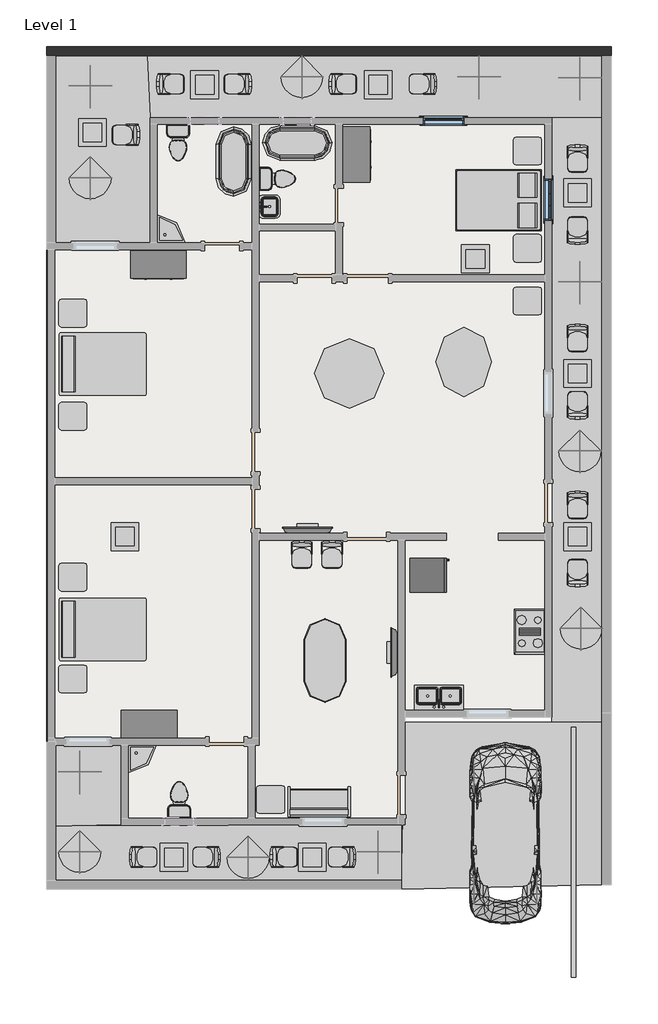
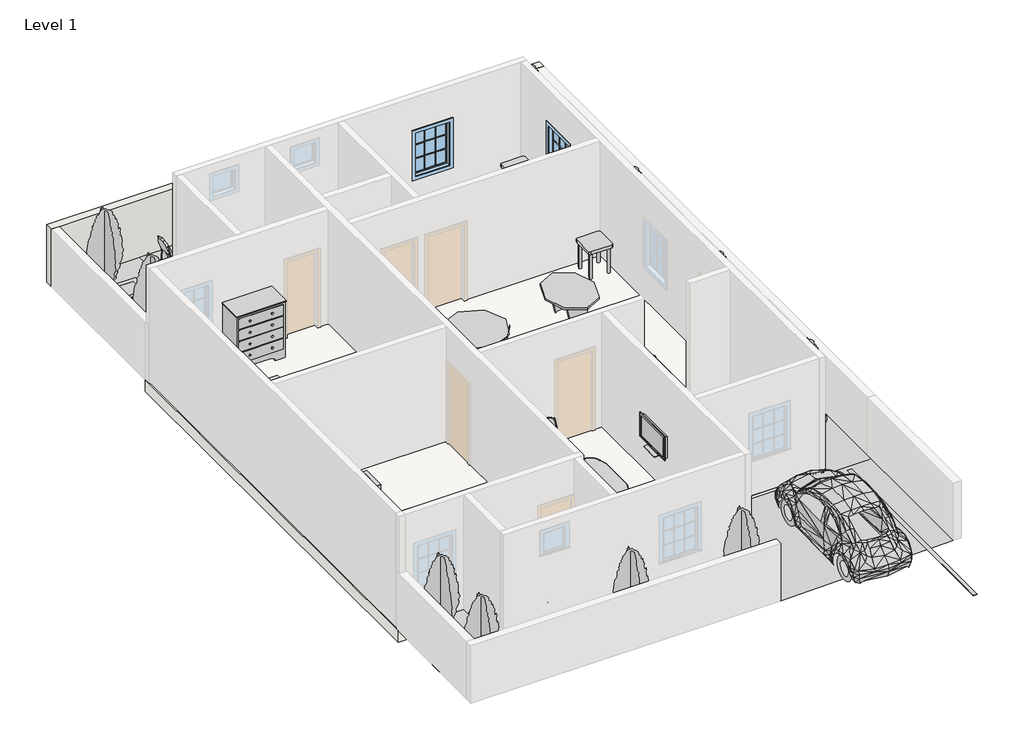
# One storey, part 2 of 2: 47 furniture elements, 12 geographic elements, 10 proxies, 9 flow terminals, 2 windows, 1 slab, 1 wall.
"""IFC4 building model written with IfcOpenShell, lengths in millimetres."""

from ifc_helpers import new_model, si_unit, frame, origin, place, context, project, spatial, polyline, outline, extrude, faceted_brep, triangles, transform, mapped, element, save
from components import proxy_bb1e6e30, parking_space_9_x_18_90_deg_b8b21359, rpc_beetle_rpc_beetle_3ce7ba48, proxy_a13a33b2, flow_terminal_bd5cdcf8, flow_terminal_a53be723, flow_terminal_62a433f7, toilet_domestic_3d_toilet_domestic_3d_f7549cf7, toilet_domestic_3d_toilet_domestic_3d_183bbd19, flow_terminal_b374fae2, furniture_c8abb964, furniture_0253826f, furniture_2babcf72, furniture_3d1d9cbc, furniture_22419f35, furniture_7a3aaa4f, furniture_b5c51a22, furniture_2c34a4f9, furniture_bbcc68ce, furniture_743965d2, furniture_bcf351fa, rpc_tree_conifer_chinese_juniper_7_1b9786cd, window_5c190c7e

model = new_model("IFC4")

# Units and contexts
model_context = context("Model", 3, world=origin())
ifc_project = project(units=[si_unit("LENGTHUNIT", "METRE", prefix="MILLI")], contexts=[model_context])

# Site, building, storey
site = spatial("IfcSite", under=ifc_project)
building = spatial("IfcBuilding", under=site)
storey = spatial("IfcBuildingStorey", under=building, Name="Level 1", Elevation=0.0)

# Proxies
placement = place(None, origin())
element("IfcBuildingElementProxy", 1, Name="Building Element Proxy", at=placement, inside=storey, context=model_context, shape_type="Tessellation", body=[
    triangles([(-15821.9726166, -3813.3326454, 0.0), (-14178.8159363, -3813.3326454, 0.0), (-14178.8159363, -5565.9329361, 0.0), (-15821.9726166, -5591.5796265, 0.0)], [[1, 4, 3], [3, 2, 1]], closed=False),
])
element("IfcBuildingElementProxy", 2, Name="Building Element Proxy", at=placement, inside=storey, context=model_context, shape_type="Tessellation", body=[
    triangles([(-13543.8163239, 7210.2674515, 0.0), (-15618.772229, 7210.2674515, 0.0), (-15618.772229, 11307.1063385, 0.0), (-13609.6855591, 11307.1063385, 0.0), (-13543.8163239, 9953.4668701, 0.0)], [[3, 2, 5], [3, 5, 4], [5, 2, 1]], closed=False),
])
element("IfcBuildingElementProxy", 3, Name="Building Element Proxy", at=placement, inside=storey, context=model_context, shape_type="Tessellation", body=[
    triangles([(-13528.6928284, 11219.4930817, 0.0), (-13558.0142944, 11217.5536652, 0.0), (-13543.8163239, 9953.4668701, 0.0), (-3629.9726166, 11225.4520203, 0.0), (-3629.9726166, 9951.5193146, 0.0), (-3629.9726166, 11307.1063385, 0.0), (-13621.8266785, 11226.9228607, 0.0), (-13607.6345215, 11233.7224457, 0.0), (-13588.6101013, 9952.7145905, 0.0), (-13611.7633392, 9956.2806519, 0.0), (-8604.8497696, 11307.1063385, 0.0), (-13593.9981445, 11307.1063385, 0.0)], [[2, 10, 3], [3, 10, 9], [10, 2, 7], [7, 8, 12], [8, 7, 2], [12, 8, 2], [2, 1, 12], [1, 3, 11], [5, 3, 9], [11, 3, 5], [3, 1, 2], [11, 4, 6], [4, 11, 5], [1, 11, 12]], closed=False),
])
element("IfcBuildingElementProxy", 4, Name="Building Element Proxy", at=placement, inside=storey, context=model_context, shape_type="Tessellation", body=[
    triangles([(-4730.0159363, 9953.4668701, 0.0), (-3629.9726166, 9959.906012, 0.0), (-4730.0159363, -3203.7326454, 0.0), (-3629.9726166, -3120.094146, 0.0), (-4724.8371826, -3329.7798935, 0.0), (-3629.9726166, -3346.9826225, 0.0)], [[4, 1, 3], [6, 3, 5], [4, 2, 1], [6, 4, 3]], closed=False),
])
element("IfcBuildingElementProxy", 5, Name="Building Element Proxy", at=placement, inside=storey, context=model_context, shape_type="Tessellation", body=[
    triangles([(-15618.772229, -5583.4679123, 0.0), (-14133.7047363, -5661.9735855, 0.0), (-15618.772229, -6777.6938553, 0.0), (-8032.0161301, -6777.6938553, 0.0), (-8032.0161301, -5565.9329361, 0.0)], [[1, 3, 2], [2, 4, 5], [4, 2, 3], [2, 5, 1]], closed=False),
])
element("IfcBuildingElementProxy", 6, Name="Building Element Proxy", at=placement, inside=storey, context=model_context, shape_type="Tessellation", body=[
    triangles([(-7762.1273712, -3550.9722061, 0.0), (-8032.0161301, -6980.8942429, 0.0), (-3629.9726166, -6879.2940491, 0.0), (-3629.9726166, -3374.0021942, 0.0), (-4730.0653519, -3327.8820442, 0.0), (-3629.9726166, -3308.4620087, 0.0), (-3629.9726166, -3320.1990829, 0.0), (-7860.2021988, -3759.4240173, 0.0), (-7955.8161301, -3309.578801, 0.0)], [[2, 8, 9], [1, 8, 5], [9, 1, 5], [1, 9, 8], [8, 2, 5], [3, 4, 5], [5, 6, 9], [5, 7, 6], [7, 5, 4], [3, 5, 2]], closed=False),
])
proxy_shape = proxy_bb1e6e30(model_context)
element("IfcBuildingElementProxy", 7, Name="Cook Top-4 Unit : 36\" x 20\"", ObjectType="Cook Top-4 Unit : 36\" x 20\"", at=placement, inside=storey, context=model_context, shape_type="MappedRepresentation", body=[
    mapped(proxy_shape, transform((-5212.6159934, -1324.1326671, 0.0), x_axis=(0.0, -1.0000000000000004, 0.0), y_axis=(1.0000000000000004, 0.0, 0.0), z_axis=(0.0, 0.0, 1.0))),
])
parking_space_9_x_18_90_deg_shape = parking_space_9_x_18_90_deg_b8b21359(model_context)
element("IfcBuildingElementProxy", 8, Name="Parking Space : 9' x 18' - 90 deg", ObjectType="Parking Space : 9' x 18' - 90 deg", at=placement, inside=storey, context=model_context, shape_type="MappedRepresentation", body=[
    mapped(parking_space_9_x_18_90_deg_shape, transform((-4247.4159934, -8911.2940071, 0.0), x_axis=(-1.0000000000000004, 0.0, 0.0), y_axis=(0.0, -1.0000000000000004, 0.0), z_axis=(0.0, 0.0, 1.0))),
])
rpc_beetle_rpc_beetle_shape = rpc_beetle_rpc_beetle_3ce7ba48(model_context)
element("IfcBuildingElementProxy", 9, Name="RPC Beetle : RPC Beetle", ObjectType="RPC Beetle : RPC Beetle", at=placement, inside=storey, context=model_context, shape_type="MappedRepresentation", body=[
    mapped(rpc_beetle_rpc_beetle_shape, transform((-5746.0159934, -6980.8940071, 0.0), x_axis=(1.0, 0.0, 0.0), y_axis=(0.0, 1.0, 0.0), z_axis=(0.0, 0.0, 1.0))),
])
proxy_2_shape = proxy_a13a33b2(model_context)
element("IfcBuildingElementProxy", 10, Name="Refrigerator : 30\" x 32\" RH", ObjectType="Refrigerator : 30\" x 32\" RH", at=placement, inside=storey, context=model_context, shape_type="MappedRepresentation", body=[
    mapped(proxy_2_shape, transform((-7455.7534934, -87.0816386, 0.0), x_axis=(0.0, 1.0000000000000002, 0.0), y_axis=(-1.0000000000000002, 0.0, 0.0), z_axis=(0.0, 0.0, 1.0))),
])

# Flow terminals
flow_terminal_shape = flow_terminal_bd5cdcf8(model_context)
element("IfcFlowTerminal", 11, ObjectType="Sink - Corner Floor : 24\"", at=placement, inside=storey, context=model_context, shape_type="MappedRepresentation", body=[
    mapped(flow_terminal_shape, transform((-13391.4159934, 7210.2673329, 609.6), x_axis=(1.0, 0.0, 0.0), y_axis=(0.0, 1.0, 0.0), z_axis=(0.0, 0.0, 1.0))),
])
element("IfcFlowTerminal", 12, ObjectType="Sink - Corner Floor : 24\"", at=placement, inside=storey, context=model_context, shape_type="MappedRepresentation", body=[
    mapped(flow_terminal_shape, transform((-14026.4159934, -3813.3326671, 609.6), x_axis=(0.0, -1.0000000000000009, 0.0), y_axis=(1.0000000000000009, 0.0, 0.0), z_axis=(0.0, 0.0, 1.0))),
])
flow_terminal_2_shape = flow_terminal_a53be723(model_context)
element("IfcFlowTerminal", 13, ObjectType="Sink Kitchen-Double : 42\" x 21\"", at=placement, inside=storey, context=model_context, shape_type="MappedRepresentation", body=[
    mapped(flow_terminal_2_shape, transform((-7190.8267528, -2769.587266, 0.0), x_axis=(-1.0000000000000004, 0.0, 0.0), y_axis=(0.0, -1.0000000000000004, 0.0), z_axis=(0.0, 0.0, 1.0))),
])
flow_terminal_3_shape = flow_terminal_62a433f7(model_context)
element("IfcFlowTerminal", 14, ObjectType="Sink Vanity-Square : 20\" x 18\"", at=placement, inside=storey, context=model_context, shape_type="MappedRepresentation", body=[
    mapped(flow_terminal_3_shape, transform((-10976.0705923, 7981.9780923, 0.0), x_axis=(0.0, 1.0, 0.0), y_axis=(-1.0, 0.0, 0.0), z_axis=(0.0, 0.0, 1.0))),
])
toilet_domestic_3d_toilet_domestic_3d_shape = toilet_domestic_3d_toilet_domestic_3d_f7549cf7(model_context)
toilet_domestic_3d_toilet_domestic_3d_2_shape = toilet_domestic_3d_toilet_domestic_3d_183bbd19(model_context)
element("IfcFlowTerminal", 15, ObjectType="Toilet-Domestic-3D : Toilet-Domestic-3D", at=placement, inside=storey, context=model_context, shape_type="MappedRepresentation", body=[
    mapped(toilet_domestic_3d_toilet_domestic_3d_shape, transform((-12934.2159934, 9306.3713055, 0.0), x_axis=(1.0, 0.0, 0.0), y_axis=(0.0, 1.0, 0.0), z_axis=(0.0, 0.0, 1.0))),
    mapped(toilet_domestic_3d_toilet_domestic_3d_2_shape, transform((-12934.2159934, 9306.3713055, 0.0), x_axis=(1.0, 0.0, 0.0), y_axis=(0.0, 1.0, 0.0), z_axis=(0.0, 0.0, 1.0))),
])
element("IfcFlowTerminal", 16, ObjectType="Toilet-Domestic-3D : Toilet-Domestic-3D", at=placement, inside=storey, context=model_context, shape_type="MappedRepresentation", body=[
    mapped(toilet_domestic_3d_toilet_domestic_3d_shape, transform((-10661.519966, 8607.2673329, 0.0), x_axis=(0.0, 1.0000000000000002, 0.0), y_axis=(-1.0000000000000002, 0.0, 0.0), z_axis=(0.0, 0.0, 1.0))),
    mapped(toilet_domestic_3d_toilet_domestic_3d_2_shape, transform((-10661.519966, 8607.2673329, 0.0), x_axis=(0.0, 1.0000000000000002, 0.0), y_axis=(-1.0000000000000002, 0.0, 0.0), z_axis=(0.0, 0.0, 1.0))),
])
element("IfcFlowTerminal", 17, ObjectType="Toilet-Domestic-3D : Toilet-Domestic-3D", at=placement, inside=storey, context=model_context, shape_type="MappedRepresentation", body=[
    mapped(toilet_domestic_3d_toilet_domestic_3d_shape, transform((-12908.8159934, -4918.8366398, 0.0), x_axis=(-0.9999999999999998, 0.0, 0.0), y_axis=(0.0, -0.9999999999999998, 0.0), z_axis=(0.0, 0.0, 1.0))),
    mapped(toilet_domestic_3d_toilet_domestic_3d_2_shape, transform((-12908.8159934, -4918.8366398, 0.0), x_axis=(-0.9999999999999998, 0.0, 0.0), y_axis=(0.0, -0.9999999999999998, 0.0), z_axis=(0.0, 0.0, 1.0))),
])
flow_terminal_4_shape = flow_terminal_b374fae2(model_context)
element("IfcFlowTerminal", 18, ObjectType="Tub-Free Standing-3D : 30\" x 60\"", at=placement, inside=storey, context=model_context, shape_type="MappedRepresentation", body=[
    mapped(flow_terminal_4_shape, transform((-11715.0159934, 8988.2673329, 0.0), x_axis=(1.0, 0.0, 0.0), y_axis=(0.0, 1.0, 0.0), z_axis=(0.0, 0.0, 1.0))),
])
element("IfcFlowTerminal", 19, ObjectType="Tub-Free Standing-3D : 30\" x 60\"", at=placement, inside=storey, context=model_context, shape_type="MappedRepresentation", body=[
    mapped(flow_terminal_4_shape, transform((-10318.0159934, 9394.6673329, 0.0), x_axis=(0.0, 1.0, 0.0), y_axis=(-1.0, 0.0, 0.0), z_axis=(0.0, 0.0, 1.0))),
])

# Furniture
furniture_shape = furniture_c8abb964(model_context)
element("IfcFurniture", 20, ObjectType="Bed-Box : Double 53\" x 74\"", at=placement, inside=storey, context=model_context, shape_type="MappedRepresentation", body=[
    mapped(furniture_shape, transform((-5663.9864852, 8476.5197919, 0.0), x_axis=(0.0, -1.0000000000000004, 0.0), y_axis=(1.0000000000000004, 0.0, 0.0), z_axis=(0.0, 0.0, 1.0))),
])
furniture_2_shape = furniture_0253826f(model_context)
element("IfcFurniture", 21, ObjectType="Bed-Standard : Double 54\" x 75\"", at=placement, inside=storey, context=model_context, shape_type="MappedRepresentation", body=[
    mapped(furniture_2_shape, transform((-14635.6677866, -1544.8211917, 0.0), x_axis=(0.0, 1.0000000000000002, 0.0), y_axis=(-1.0000000000000002, 0.0, 0.0), z_axis=(0.0, 0.0, 1.0))),
])
element("IfcFurniture", 22, ObjectType="Bed-Standard.0001 : Double 54\" x 75\"", at=placement, inside=storey, context=model_context, shape_type="MappedRepresentation", body=[
    mapped(furniture_2_shape, transform((-14635.6677866, 4271.7788083, 0.0), x_axis=(0.0, 1.0, 0.0), y_axis=(-1.0, 0.0, 0.0), z_axis=(0.0, 0.0, 1.0))),
])
furniture_3_shape = furniture_2babcf72(model_context)
element("IfcFurniture", 23, ObjectType="Dresser : 48\" x 60\" x 24\"", at=placement, inside=storey, context=model_context, shape_type="MappedRepresentation", body=[
    mapped(furniture_3_shape, transform((-9385.7789475, 9409.8605927, 0.0), x_axis=(0.0, 1.0, 0.0), y_axis=(-1.0, 0.0, 0.0), z_axis=(0.0, 0.0, 1.0))),
])
element("IfcFurniture", 24, ObjectType="Dresser : 48\" x 60\" x 24\"", at=placement, inside=storey, context=model_context, shape_type="MappedRepresentation", body=[
    mapped(furniture_3_shape, transform((-13096.8227336, 7090.830287, 0.0), x_axis=(1.0, 0.0, 0.0), y_axis=(0.0, 1.0, 0.0), z_axis=(0.0, 0.0, 1.0))),
])
element("IfcFurniture", 25, ObjectType="Dresser : 48\" x 60\" x 24\"", at=placement, inside=storey, context=model_context, shape_type="MappedRepresentation", body=[
    mapped(furniture_3_shape, transform((-13300.0227336, -2992.969713, 0.0), x_axis=(1.0, 0.0, 0.0), y_axis=(0.0, 1.0, 0.0), z_axis=(0.0, 0.0, 1.0))),
])
furniture_4_shape = furniture_3d1d9cbc(model_context)
element("IfcFurniture", 26, ObjectType="Seating-Auditorium : 18\" x 24\" x 30\"", at=placement, inside=storey, context=model_context, shape_type="MappedRepresentation", body=[
    mapped(furniture_4_shape, transform((-9395.2881245, 567.5427427, 0.0), x_axis=(-1.0000000000000002, 0.0, 0.0), y_axis=(0.0, -1.0000000000000002, 0.0), z_axis=(0.0, 0.0, 1.0))),
])
element("IfcFurniture", 27, ObjectType="Seating-Auditorium : 18\" x 24\" x 30\"", at=placement, inside=storey, context=model_context, shape_type="MappedRepresentation", body=[
    mapped(furniture_4_shape, transform((-10055.6881245, 567.5427427, 0.0), x_axis=(-1.0, 0.0, 0.0), y_axis=(0.0, -1.0, 0.0), z_axis=(0.0, 0.0, 1.0))),
])
element("IfcFurniture", 28, ObjectType="Seating-Auditorium : 18\" x 24\" x 30\"", at=placement, inside=storey, context=model_context, shape_type="MappedRepresentation", body=[
    mapped(furniture_4_shape, transform((-13899.6939644, -6108.9661382, 0.0), x_axis=(0.0, -1.0, 0.0), y_axis=(1.0, 0.0, 0.0), z_axis=(0.0, 0.0, 1.0))),
])
element("IfcFurniture", 29, ObjectType="Seating-Auditorium : 18\" x 24\" x 30\"", at=placement, inside=storey, context=model_context, shape_type="MappedRepresentation", body=[
    mapped(furniture_4_shape, transform((-12109.3405836, -6430.4218759, 0.0), x_axis=(0.0, 1.0, 0.0), y_axis=(-1.0, 0.0, 0.0), z_axis=(0.0, 0.0, 1.0))),
])
element("IfcFurniture", 30, ObjectType="Seating-Auditorium : 18\" x 24\" x 30\"", at=placement, inside=storey, context=model_context, shape_type="MappedRepresentation", body=[
    mapped(furniture_4_shape, transform((-10812.6914032, -6108.9661382, 0.0), x_axis=(0.0, -1.0000000000000004, 0.0), y_axis=(1.0000000000000004, 0.0, 0.0), z_axis=(0.0, 0.0, 1.0))),
])
element("IfcFurniture", 31, ObjectType="Seating-Auditorium : 18\" x 24\" x 30\"", at=placement, inside=storey, context=model_context, shape_type="MappedRepresentation", body=[
    mapped(furniture_4_shape, transform((-9137.5405836, -6430.4218759, 0.0), x_axis=(0.0, 1.0, 0.0), y_axis=(-1.0, 0.0, 0.0), z_axis=(0.0, 0.0, 1.0))),
])
element("IfcFurniture", 32, ObjectType="Seating-Auditorium : 18\" x 24\" x 30\"", at=placement, inside=storey, context=model_context, shape_type="MappedRepresentation", body=[
    mapped(furniture_4_shape, transform((-13879.4972948, 9411.739464, 0.0), x_axis=(0.0, 1.0000000000000002, 0.0), y_axis=(-1.0000000000000002, 0.0, 0.0), z_axis=(0.0, 0.0, 1.0))),
])
element("IfcFurniture", 33, ObjectType="Seating-Auditorium : 18\" x 24\" x 30\"", at=placement, inside=storey, context=model_context, shape_type="MappedRepresentation", body=[
    mapped(furniture_4_shape, transform((-13301.8914032, 10850.7952017, 0.0), x_axis=(0.0, -1.0000000000000004, 0.0), y_axis=(1.0000000000000004, 0.0, 0.0), z_axis=(0.0, 0.0, 1.0))),
])
element("IfcFurniture", 34, ObjectType="Seating-Auditorium : 18\" x 24\" x 30\"", at=placement, inside=storey, context=model_context, shape_type="MappedRepresentation", body=[
    mapped(furniture_4_shape, transform((-11423.5405836, 10529.339464, 0.0), x_axis=(0.0, 1.0, 0.0), y_axis=(-1.0, 0.0, 0.0), z_axis=(0.0, 0.0, 1.0))),
])
element("IfcFurniture", 35, ObjectType="Seating-Auditorium : 18\" x 24\" x 30\"", at=placement, inside=storey, context=model_context, shape_type="MappedRepresentation", body=[
    mapped(furniture_4_shape, transform((-7359.5405836, 10529.339464, 0.0), x_axis=(0.0, 1.0000000000000002, 0.0), y_axis=(-1.0000000000000002, 0.0, 0.0), z_axis=(0.0, 0.0, 1.0))),
])
element("IfcFurniture", 36, ObjectType="Seating-Auditorium : 18\" x 24\" x 30\"", at=placement, inside=storey, context=model_context, shape_type="MappedRepresentation", body=[
    mapped(furniture_4_shape, transform((-9517.2914032, 10850.7952017, 0.0), x_axis=(0.0, -1.0, 0.0), y_axis=(1.0, 0.0, 0.0), z_axis=(0.0, 0.0, 1.0))),
])
element("IfcFurniture", 37, ObjectType="Seating-Auditorium : 18\" x 24\" x 30\"", at=placement, inside=storey, context=model_context, shape_type="MappedRepresentation", body=[
    mapped(furniture_4_shape, transform((-4002.6448358, 9254.3427427, 0.0), x_axis=(-1.0000000000000002, 0.0, 0.0), y_axis=(0.0, -1.0000000000000002, 0.0), z_axis=(0.0, 0.0, 1.0))),
])
element("IfcFurniture", 38, ObjectType="Seating-Auditorium : 18\" x 24\" x 30\"", at=placement, inside=storey, context=model_context, shape_type="MappedRepresentation", body=[
    mapped(furniture_4_shape, transform((-4324.1005735, 7274.391923, 0.0), x_axis=(1.0000000000000002, 0.0, 0.0), y_axis=(0.0, 1.0000000000000002, 0.0), z_axis=(0.0, 0.0, 1.0))),
])
element("IfcFurniture", 39, ObjectType="Seating-Auditorium : 18\" x 24\" x 30\"", at=placement, inside=storey, context=model_context, shape_type="MappedRepresentation", body=[
    mapped(furniture_4_shape, transform((-4002.6448358, 5317.3427427, 0.0), x_axis=(-1.0000000000000002, 0.0, 0.0), y_axis=(0.0, -1.0000000000000002, 0.0), z_axis=(0.0, 0.0, 1.0))),
])
element("IfcFurniture", 40, ObjectType="Seating-Auditorium : 18\" x 24\" x 30\"", at=placement, inside=storey, context=model_context, shape_type="MappedRepresentation", body=[
    mapped(furniture_4_shape, transform((-4324.1005735, 3438.991923, 0.0), x_axis=(1.0000000000000002, 0.0, 0.0), y_axis=(0.0, 1.0000000000000002, 0.0), z_axis=(0.0, 0.0, 1.0))),
])
element("IfcFurniture", 41, ObjectType="Seating-Auditorium : 18\" x 24\" x 30\"", at=placement, inside=storey, context=model_context, shape_type="MappedRepresentation", body=[
    mapped(furniture_4_shape, transform((-4002.6448358, 1653.3927427, 0.0), x_axis=(-1.0000000000000004, 0.0, 0.0), y_axis=(0.0, -1.0000000000000004, 0.0), z_axis=(0.0, 0.0, 1.0))),
])
element("IfcFurniture", 42, ObjectType="Seating-Auditorium : 18\" x 24\" x 30\"", at=placement, inside=storey, context=model_context, shape_type="MappedRepresentation", body=[
    mapped(furniture_4_shape, transform((-4324.1005735, -236.5694169, 0.0), x_axis=(1.0000000000000004, 0.0, 0.0), y_axis=(0.0, 1.0000000000000004, 0.0), z_axis=(0.0, 0.0, 1.0))),
])
furniture_5_shape = furniture_22419f35(model_context)
element("IfcFurniture", 43, ObjectType="Sofa : 54\"", at=placement, inside=storey, context=model_context, shape_type="MappedRepresentation", body=[
    mapped(furniture_5_shape, transform((-9765.0455016, -4911.7785688, 0.0), x_axis=(-1.0, 0.0, 0.0), y_axis=(0.0, -1.0, 0.0), z_axis=(0.0, 0.0, 1.0))),
])
furniture_6_shape = furniture_7a3aaa4f(model_context)
element("IfcFurniture", 44, ObjectType="TV - Flat Screen : 42\"", at=placement, inside=storey, context=model_context, shape_type="MappedRepresentation", body=[
    mapped(furniture_6_shape, transform((-10093.3605075, 893.4059565, 914.4), x_axis=(-1.0000000000000004, 0.0, 0.0), y_axis=(0.0, -1.0000000000000004, 0.0), z_axis=(0.0, 0.0, 1.0))),
])
element("IfcFurniture", 45, ObjectType="TV - Flat Screen : 42\"", at=placement, inside=storey, context=model_context, shape_type="MappedRepresentation", body=[
    mapped(furniture_6_shape, transform((-8192.154617, -1785.2771813, 914.4), x_axis=(0.0, -1.0000000000000004, 0.0), y_axis=(1.0000000000000004, 0.0, 0.0), z_axis=(0.0, 0.0, 1.0))),
])
furniture_7_shape = furniture_b5c51a22(model_context)
element("IfcFurniture", 46, ObjectType="Table-Coffee : 24\" x 24\" x 24\"", at=placement, inside=storey, context=model_context, shape_type="MappedRepresentation", body=[
    mapped(furniture_7_shape, transform((-14120.8817601, 663.4562551, 0.0), x_axis=(1.0, 0.0, 0.0), y_axis=(0.0, 1.0, 0.0), z_axis=(0.0, 0.0, 1.0))),
])
element("IfcFurniture", 47, ObjectType="Table-Coffee : 24\" x 24\" x 24\"", at=placement, inside=storey, context=model_context, shape_type="MappedRepresentation", body=[
    mapped(furniture_7_shape, transform((-6424.6817601, 6759.4562551, 0.0), x_axis=(1.0, 0.0, 0.0), y_axis=(0.0, 1.0, 0.0), z_axis=(0.0, 0.0, 1.0))),
])
element("IfcFurniture", 48, ObjectType="Table-Coffee : 24\" x 24\" x 24\"", at=placement, inside=storey, context=model_context, shape_type="MappedRepresentation", body=[
    mapped(furniture_7_shape, transform((-13042.2843213, -6372.3437449, 0.0), x_axis=(1.0, 0.0, 0.0), y_axis=(0.0, 1.0, 0.0), z_axis=(0.0, 0.0, 1.0))),
])
element("IfcFurniture", 49, ObjectType="Table-Coffee : 24\" x 24\" x 24\"", at=placement, inside=storey, context=model_context, shape_type="MappedRepresentation", body=[
    mapped(furniture_7_shape, transform((-10006.0817601, -6372.3437449, 0.0), x_axis=(1.0, 0.0, 0.0), y_axis=(0.0, 1.0, 0.0), z_axis=(0.0, 0.0, 1.0))),
])
element("IfcFurniture", 50, ObjectType="Table-Coffee : 24\" x 24\" x 24\"", at=placement, inside=storey, context=model_context, shape_type="MappedRepresentation", body=[
    mapped(furniture_7_shape, transform((-14832.0817601, 9528.0562551, 0.0), x_axis=(1.0, 0.0, 0.0), y_axis=(0.0, 1.0, 0.0), z_axis=(0.0, 0.0, 1.0))),
])
element("IfcFurniture", 51, ObjectType="Table-Coffee : 24\" x 24\" x 24\"", at=placement, inside=storey, context=model_context, shape_type="MappedRepresentation", body=[
    mapped(furniture_7_shape, transform((-12368.2817601, 10576.8949151, 0.0), x_axis=(1.0, 0.0, 0.0), y_axis=(0.0, 1.0, 0.0), z_axis=(0.0, 0.0, 1.0))),
])
element("IfcFurniture", 52, ObjectType="Table-Coffee : 24\" x 24\" x 24\"", at=placement, inside=storey, context=model_context, shape_type="MappedRepresentation", body=[
    mapped(furniture_7_shape, transform((-8558.2817601, 10576.8949151, 0.0), x_axis=(1.0, 0.0, 0.0), y_axis=(0.0, 1.0, 0.0), z_axis=(0.0, 0.0, 1.0))),
])
element("IfcFurniture", 53, ObjectType="Table-Coffee : 24\" x 24\" x 24\"", at=placement, inside=storey, context=model_context, shape_type="MappedRepresentation", body=[
    mapped(furniture_7_shape, transform((-4181.6384713, 8207.2562551, 0.0), x_axis=(1.0, 0.0, 0.0), y_axis=(0.0, 1.0, 0.0), z_axis=(0.0, 0.0, 1.0))),
])
element("IfcFurniture", 54, ObjectType="Table-Coffee : 24\" x 24\" x 24\"", at=placement, inside=storey, context=model_context, shape_type="MappedRepresentation", body=[
    mapped(furniture_7_shape, transform((-4181.6384713, 4244.8562551, 0.0), x_axis=(1.0, 0.0, 0.0), y_axis=(0.0, 1.0, 0.0), z_axis=(0.0, 0.0, 1.0))),
])
element("IfcFurniture", 55, ObjectType="Table-Coffee : 24\" x 24\" x 24\"", at=placement, inside=storey, context=model_context, shape_type="MappedRepresentation", body=[
    mapped(furniture_7_shape, transform((-4181.6384713, 663.4562551, 0.0), x_axis=(1.0, 0.0, 0.0), y_axis=(0.0, 1.0, 0.0), z_axis=(0.0, 0.0, 1.0))),
])
furniture_8_shape = furniture_2c34a4f9(model_context)
element("IfcFurniture", 56, ObjectType="Table-Dining Oval : 36\" x 72\"", at=placement, inside=storey, context=model_context, shape_type="MappedRepresentation", body=[
    mapped(furniture_8_shape, transform((-10066.514354, -1557.312995, 0.0), x_axis=(0.0, 1.0, 0.0), y_axis=(-1.0, 0.0, 0.0), z_axis=(0.0, 0.0, 1.0))),
])
furniture_9_shape = furniture_bbcc68ce(model_context)
element("IfcFurniture", 57, ObjectType="Table-Dining Round w Chairs : 60\" Diameter", at=placement, inside=storey, context=model_context, shape_type="MappedRepresentation", body=[
    mapped(furniture_9_shape, transform((-9278.6979606, 4524.9460214, 0.0), x_axis=(1.0, 0.0, 0.0), y_axis=(0.0, 1.0, 0.0), z_axis=(0.0, 0.0, 1.0))),
])
furniture_10_shape = furniture_743965d2(model_context)
element("IfcFurniture", 58, ObjectType="Table-Ellipse : 60\" x 48\"", at=placement, inside=storey, context=model_context, shape_type="MappedRepresentation", body=[
    mapped(furniture_10_shape, transform((-6660.4159934, 4594.0673329, 0.0), x_axis=(0.0, 1.0000000000000002, 0.0), y_axis=(-1.0000000000000002, 0.0, 0.0), z_axis=(0.0, 0.0, 1.0))),
])
furniture_11_shape = furniture_bcf351fa(model_context)
element("IfcFurniture", 59, ObjectType="Table-End : 24\" x 24\"", at=placement, inside=storey, context=model_context, shape_type="MappedRepresentation", body=[
    mapped(furniture_11_shape, transform((-5571.9496237, 6930.8673329, 0.0), x_axis=(1.0, 0.0, 0.0), y_axis=(0.0, 1.0, 0.0), z_axis=(0.0, 0.0, 1.0))),
])
element("IfcFurniture", 60, ObjectType="Table-End : 24\" x 24\"", at=placement, inside=storey, context=model_context, shape_type="MappedRepresentation", body=[
    mapped(furniture_11_shape, transform((-5571.9496237, 9064.4673329, 0.0), x_axis=(1.0, 0.0, 0.0), y_axis=(0.0, 1.0, 0.0), z_axis=(0.0, 0.0, 1.0))),
])
element("IfcFurniture", 61, ObjectType="Table-End : 24\" x 24\"", at=placement, inside=storey, context=model_context, shape_type="MappedRepresentation", body=[
    mapped(furniture_11_shape, transform((-15554.1496237, 5508.4673329, 0.0), x_axis=(1.0, 0.0, 0.0), y_axis=(0.0, 1.0, 0.0), z_axis=(0.0, 0.0, 1.0))),
])
element("IfcFurniture", 62, ObjectType="Table-End : 24\" x 24\"", at=placement, inside=storey, context=model_context, shape_type="MappedRepresentation", body=[
    mapped(furniture_11_shape, transform((-15554.1496237, 3247.8673329, 0.0), x_axis=(1.0, 0.0, 0.0), y_axis=(0.0, 1.0, 0.0), z_axis=(0.0, 0.0, 1.0))),
])
element("IfcFurniture", 63, ObjectType="Table-End : 24\" x 24\"", at=placement, inside=storey, context=model_context, shape_type="MappedRepresentation", body=[
    mapped(furniture_11_shape, transform((-15554.1496237, -282.7326671, 0.0), x_axis=(1.0, 0.0, 0.0), y_axis=(0.0, 1.0, 0.0), z_axis=(0.0, 0.0, 1.0))),
])
element("IfcFurniture", 64, ObjectType="Table-End : 24\" x 24\"", at=placement, inside=storey, context=model_context, shape_type="MappedRepresentation", body=[
    mapped(furniture_11_shape, transform((-15554.1496237, -2517.9326671, 0.0), x_axis=(1.0, 0.0, 0.0), y_axis=(0.0, 1.0, 0.0), z_axis=(0.0, 0.0, 1.0))),
])
element("IfcFurniture", 65, ObjectType="Table-End : 24\" x 24\"", at=placement, inside=storey, context=model_context, shape_type="MappedRepresentation", body=[
    mapped(furniture_11_shape, transform((-5571.9496237, 5775.1673329, 0.0), x_axis=(1.0, 0.0, 0.0), y_axis=(0.0, 1.0, 0.0), z_axis=(0.0, 0.0, 1.0))),
])
element("IfcFurniture", 66, ObjectType="Table-End : 24\" x 24\"", at=placement, inside=storey, context=model_context, shape_type="MappedRepresentation", body=[
    mapped(furniture_11_shape, transform((-11210.7496237, -5159.5326671, 0.0), x_axis=(1.0, 0.0, 0.0), y_axis=(0.0, 1.0, 0.0), z_axis=(0.0, 0.0, 1.0))),
])

# Geographic elements
rpc_tree_conifer_chinese_juniper_7_shape = rpc_tree_conifer_chinese_juniper_7_1b9786cd(model_context)
element("IfcGeographicElement", 67, ObjectType="RPC Tree - Conifer : Chinese Juniper - 7'", at=placement, inside=storey, context=model_context, shape_type="MappedRepresentation", body=[
    mapped(rpc_tree_conifer_chinese_juniper_7_shape, transform((-15093.4126645, -4397.5326671, 0.0), x_axis=(1.0, 0.0, 0.0), y_axis=(0.0, 1.0, 0.0), z_axis=(0.0, 0.0, 1.0))),
])
element("IfcGeographicElement", 68, ObjectType="RPC Tree - Conifer : Chinese Juniper - 7'", at=placement, inside=storey, context=model_context, shape_type="MappedRepresentation", body=[
    mapped(rpc_tree_conifer_chinese_juniper_7_shape, transform((-15093.4126645, -6150.1326671, 0.0), x_axis=(1.0, 0.0, 0.0), y_axis=(0.0, 1.0, 0.0), z_axis=(0.0, 0.0, 1.0))),
])
element("IfcGeographicElement", 69, ObjectType="RPC Tree - Conifer : Chinese Juniper - 7'", at=placement, inside=storey, context=model_context, shape_type="MappedRepresentation", body=[
    mapped(rpc_tree_conifer_chinese_juniper_7_shape, transform((-11398.6152257, -6277.1326671, 0.0), x_axis=(1.0, 0.0, 0.0), y_axis=(0.0, 1.0, 0.0), z_axis=(0.0, 0.0, 1.0))),
])
element("IfcGeographicElement", 70, ObjectType="RPC Tree - Conifer : Chinese Juniper - 7'", at=placement, inside=storey, context=model_context, shape_type="MappedRepresentation", body=[
    mapped(rpc_tree_conifer_chinese_juniper_7_shape, transform((-8540.2126645, -6150.1326671, 0.0), x_axis=(1.0, 0.0, 0.0), y_axis=(0.0, 1.0, 0.0), z_axis=(0.0, 0.0, 1.0))),
])
element("IfcGeographicElement", 71, ObjectType="RPC Tree - Conifer : Chinese Juniper - 7'", at=placement, inside=storey, context=model_context, shape_type="MappedRepresentation", body=[
    mapped(rpc_tree_conifer_chinese_juniper_7_shape, transform((-14864.8126645, 8632.6673329, 0.0), x_axis=(1.0, 0.0, 0.0), y_axis=(0.0, 1.0, 0.0), z_axis=(0.0, 0.0, 1.0))),
])
element("IfcGeographicElement", 72, ObjectType="RPC Tree - Conifer : Chinese Juniper - 7'", at=placement, inside=storey, context=model_context, shape_type="MappedRepresentation", body=[
    mapped(rpc_tree_conifer_chinese_juniper_7_shape, transform((-14864.8126645, 10646.7059929, 0.0), x_axis=(1.0, 0.0, 0.0), y_axis=(0.0, 1.0, 0.0), z_axis=(0.0, 0.0, 1.0))),
])
element("IfcGeographicElement", 73, ObjectType="RPC Tree - Conifer : Chinese Juniper - 7'", at=placement, inside=storey, context=model_context, shape_type="MappedRepresentation", body=[
    mapped(rpc_tree_conifer_chinese_juniper_7_shape, transform((-10216.6126645, 10849.9059929, 0.0), x_axis=(1.0, 0.0, 0.0), y_axis=(0.0, 1.0, 0.0), z_axis=(0.0, 0.0, 1.0))),
])
element("IfcGeographicElement", 74, ObjectType="RPC Tree - Conifer : Chinese Juniper - 7'", at=placement, inside=storey, context=model_context, shape_type="MappedRepresentation", body=[
    mapped(rpc_tree_conifer_chinese_juniper_7_shape, transform((-6330.4126645, 10849.9059929, 0.0), x_axis=(1.0, 0.0, 0.0), y_axis=(0.0, 1.0, 0.0), z_axis=(0.0, 0.0, 1.0))),
])
element("IfcGeographicElement", 75, ObjectType="RPC Tree - Conifer : Chinese Juniper - 7'", at=placement, inside=storey, context=model_context, shape_type="MappedRepresentation", body=[
    mapped(rpc_tree_conifer_chinese_juniper_7_shape, transform((-4112.7693757, 10824.5059929, 0.0), x_axis=(1.0, 0.0, 0.0), y_axis=(0.0, 1.0, 0.0), z_axis=(0.0, 0.0, 1.0))),
])
element("IfcGeographicElement", 76, ObjectType="RPC Tree - Conifer : Chinese Juniper - 7'", at=placement, inside=storey, context=model_context, shape_type="MappedRepresentation", body=[
    mapped(rpc_tree_conifer_chinese_juniper_7_shape, transform((-4112.7693757, 6346.6673329, 0.0), x_axis=(1.0, 0.0, 0.0), y_axis=(0.0, 1.0, 0.0), z_axis=(0.0, 0.0, 1.0))),
])
element("IfcGeographicElement", 77, ObjectType="RPC Tree - Conifer : Chinese Juniper - 7'", at=placement, inside=storey, context=model_context, shape_type="MappedRepresentation", body=[
    mapped(rpc_tree_conifer_chinese_juniper_7_shape, transform((-4112.7693757, 2638.2673329, 0.0), x_axis=(1.0, 0.0, 0.0), y_axis=(0.0, 1.0, 0.0), z_axis=(0.0, 0.0, 1.0))),
])
element("IfcGeographicElement", 78, ObjectType="RPC Tree - Conifer : Chinese Juniper - 7'", at=placement, inside=storey, context=model_context, shape_type="MappedRepresentation", body=[
    mapped(rpc_tree_conifer_chinese_juniper_7_shape, transform((-4087.3693757, -1247.9326671, 0.0), x_axis=(1.0, 0.0, 0.0), y_axis=(0.0, 1.0, 0.0), z_axis=(0.0, 0.0, 1.0))),
])

# Slab
element("IfcSlab", 79, ObjectType="Generic - 12\"", at=placement, inside=storey, context=model_context, shape_type="SweptSolid", body=[
    extrude(outline(polyline([(-13543.8159934, 7210.2673329), (-13543.8159934, 9953.4673329), (-4730.0159934, 9953.4673329), (-4730.0159934, -3203.7326671), (-7955.8159934, -3203.7326671), (-7955.8159934, -5565.9326671), (-14178.8159934, -5565.9326671), (-14178.8159934, -3813.3326671), (-15821.9727047, -3813.3326671), (-15821.9727047, 7210.2673329), (-13543.8159934, 7210.2673329)])), frame((0.0, 0.0, -304.8), z_axis=(0.0, 0.0, 1.0), x_axis=(1.0, 0.0, 0.0)), (0.0, 0.0, 1.0), 304.8),
])

# Wall
element("IfcWall", 80, ObjectType="Generic - 8\"", at=placement, inside=storey, context=model_context, shape_type="Brep", body=[
    faceted_brep([(-15821.9727047, 11307.1059929, 0.0), (-15618.7727047, 11307.1059929, 0.0), (-3629.9727047, 11307.1059929, 0.0), (-3426.7727047, 11307.1059929, 0.0), (-3426.7727047, 11307.1059929, 1524.0), (-3629.9727047, 11307.1059929, 1524.0), (-15618.7727047, 11307.1059929, 1524.0), (-15821.9727047, 11307.1059929, 1524.0), (-15821.9727047, 11510.3059929, 0.0), (-15821.9727047, 11510.3059929, 1524.0), (-3426.7727047, 11510.3059929, 1524.0), (-3426.7727047, 11510.3059929, 0.0)], [[[0, 1, 2, 3, 4, 5, 6, 7]], [[8, 9, 10, 11]], [[3, 2, 1, 0, 8, 11]], [[7, 6, 5, 4, 10, 9]], [[4, 3, 11, 10]], [[0, 7, 9, 8]]]),
])

# Windows
window_shape = window_5c190c7e(model_context)
element("IfcWindow", 81, ObjectType="Casement 3x3 with Trim : 36\" x 48\"", at=placement, inside=storey, context=model_context, shape_type="MappedRepresentation", body=[
    mapped(window_shape, transform((-7104.9159934, 9877.2673329, 0.0), x_axis=(1.0, 0.0, 0.0), y_axis=(0.0, 1.0, 0.0), z_axis=(0.0, 0.0, 1.0))),
])
element("IfcWindow", 82, ObjectType="Casement 3x3 with Trim : 36\" x 48\"", at=placement, inside=storey, context=model_context, shape_type="MappedRepresentation", body=[
    mapped(window_shape, transform((-4806.2159934, 8150.0673329, 0.0), x_axis=(0.0, -1.0, 0.0), y_axis=(1.0, 0.0, 0.0), z_axis=(0.0, 0.0, 1.0))),
])

save(model, "model.ifc")

# Revit data of these elements
# Type "Cook Top-4 Unit : 36\" x 20\""
#   Assembly Code = "E1090400"
#   Depth = 2' - 0"
#   Width = 3' - 0"
#   Burner Material = Steel, Chrome Plated
#   Cooktop Material = Steel, Polished
#   Default Elevation = 0
# Type "Parking Space : 9' x 18' - 90 deg"
#   Angle = 90.00°
#   Parking Length = 18' - 0"
#   Parking Width = 9' - 0"
#   pl = 18' - 0"
#   pw = 9' - 0"
# Type "RPC Beetle : RPC Beetle"
#   built-in parameter 1005195 = "RPC-16-0U6E-L4EG-ENH1-J3KF-SVEL-0TX4-C0"
#   Height = 0
# Type "Refrigerator : 30\" x 32\" RH"
#   Label = "REF."
#   Assembly Code = "E1090400"
#   Depth = 2' - 7 3/4"
#   Handle = 2' - 3"
#   Height = 5' - 10"
#   Rear Clearance = 0' - 2"
#   Top Door Height = 1' - 8"
#   Width = 2' - 5 3/8"
#   Material = Steel, Paint Finish, Ivory, Glossy
#   Default Elevation = 0
# Type "Sink - Corner Floor : 24\""
#   WFU = 2
#   Sink Radius = 2' - 0"
#   Sink Depth = 0' - 3 1/2"
#   Sanitary Radius = 3/4"
#   Sanitary Diameter = 1 1/2"
#   Radius 1 = 1' - 10"
#   Edge Width = 0' - 2"
#   Sink Material = none
#   HWFU = 0
#   Default Elevation = 0
#   CWFU = 0
# Type "Sink Kitchen-Double : 42\" x 21\""
#   Assembly Code = "D2010410"
#   Counter Height = 3' - 0"
#   Depth = 1' - 9"
#   Width = 3' - 6"
#   Faucet Material = Steel, Polished
#   Sink Material = Steel, Polished
#   Default Elevation = 0
# Type "Sink Vanity-Square : 20\" x 18\""
#   Assembly Code = "D2010400"
#   Counter Height = 2' - 7"
#   Depth = 1' - 6"
#   Width = 1' - 8"
#   Basin Material = Porcelain, Linen
#   Faucet Material = Steel, Polished
#   Default Elevation = 0
# Type "Toilet-Domestic-3D : Toilet-Domestic-3D"
#   Assembly Code = "D2010110"
#   Toilet - Bowl/Basin Material = Porcelain, Linen
#   Toilet - Seat Material = Laminate, Linen, Matte
#   Default Elevation = 0
# Type "Tub-Free Standing-3D : 30\" x 60\""
#   Assembly Code = "D2010110"
#   Height = 1' - 6"
#   Length = 5' - 0"
#   Width = 2' - 6"
#   Tub Material = Porcelain, Ivory
#   Default Elevation = 0
# Type "Bed-Box : Double 53\" x 74\""
#   Assembly Code = "E2020200"
#   Length = 6' - 2"
#   Width = 4' - 5"
#   Frame Material = Birch
#   Mattress Material = Linen, White
#   Default Elevation = 0
# Type "Bed-Standard : Double 54\" x 75\""
#   Assembly Code = "E2020200"
#   Length = 6' - 3"
#   Width = 4' - 6"
#   Leg Material = Steel, Chrome Plated
#   Mattress Material = Linen, White
#   Default Elevation = 0
# Type "Bed-Standard.0001 : Double 54\" x 75\""
#   Assembly Code = "E2020200"
#   Length = 6' - 3"
#   Width = 4' - 6"
#   Leg Material = Steel, Chrome Plated
#   Mattress Material = Linen, White
#   Default Elevation = 0
# Type "Dresser : 48\" x 60\" x 24\""
#   Assembly Code = "E2020200"
#   Depth = 2' - 0"
#   Height = 5' - 0"
#   Width = 4' - 0"
#   Dresser Material = Laminate - Ivory, Glossy
#   Drawer Material = Laminate, Ivory, Matte
#   Knob Material = Cherry
#   Default Elevation = 0
# Type "Seating-Auditorium : 18\" x 24\" x 30\""
#   Assembly Code = "E2020200"
#   Seat Material = Linen, Beige
#   Frame Material = Steel, Paint Finish, Dark Gray, Matte
#   Default Elevation = 0
# Type "Sofa : 54\""
#   Assembly Code = "E2020200"
#   Width = 4' - 6"
#   Seat Material = none
#   Frame Material = none
#   Default Elevation = 0
# Type "TV - Flat Screen : 42\""
#   SinAng = 0' - 0.0193"
#   L = 3' - 0.71517"
#   H = 1' - 8.65418"
#   Thickness = 0' - 4.33071"
#   Diagonal = 3' - 6.12598"
#   CosAng = 0' - 0.03431"
#   Stand [instance default] = yes
#   Default Elevation = 0
# Type "Table-Coffee : 24\" x 24\" x 24\""
#   Assembly Code = "E2020200"
#   Height = 2' - 0"
#   Length = 2' - 0"
#   Width = 2' - 0"
#   Top Material = none
#   Frame Material = none
#   Default Elevation = 0
# Type "Table-Dining Oval : 36\" x 72\""
#   Assembly Code = "E2020200"
#   Length = 6' - 0"
#   Width = 3' - 0"
#   Base Material = Steel, Chrome Plated
#   Top Material = Glass - Clear, Grey
#   Default Elevation = 0
#   Description = (empty or 0)
# Type "Table-Dining Round w Chairs : 60\" Diameter"
#   Assembly Code = "E2020200"
#   Radius = 2' - 6"
#   Diameter = 5' - 0"
#   Height = 2' - 6"
#   Chairs = 6
#   Base Material = Pine
#   Top Material = Laminate, Linen, Matte
#   Default Elevation = 0
# Type "Table-Ellipse : 60\" x 48\""
#   Assembly Code = "E2020200"
#   Half Width = 2' - 0"
#   Half Length = 2' - 6"
#   Height = 2' - 6"
#   Length = 5' - 0"
#   Width = 4' - 0"
#   Base Material = Birch
#   Top Material = Birch
#   Default Elevation = 0
# Type "Table-End : 24\" x 24\""
#   Assembly Code = "E2020200"
#   Height = 2' - 6"
#   Length = 2' - 0"
#   Width = 2' - 0"
#   Base Material = Birch
#   Top Material = Laminate, Ivory, Matte
#   Default Elevation = 0
# Type "RPC Tree - Conifer : Chinese Juniper - 7'"
#   built-in parameter 1005198 = "{2, 15},{39, RPC-16-FUM3-UUQ0-UBF0-N000-ST1L-LVER-AU},{1, 0},{1, 0},{2, 13},{1, 8},{5, Color},{1, 0},{1, 0},{3, 0.8},{3, 0.8},{3, 0.8},{1, 8},{7, BBoxMin},{1, 0},{1, 0},{1, 0},{1, 0},{1, 0},{1, 8},{7, BBoxMax},{1, 0},{1, 0},{1, 0},{1, 0},{1, 0},{2, 11},{9, RPCTypeId},{1, 0},{1, 0},{39, RPC-16-FUM3-UUQ0-UBF0-N000-ST1L-LVER-AU},{1, 6},{14, RPCPlantHeight},{1, 0},{1, 0},{1, 7},{2, 11},{7, keyword},{1, 0},{1, 0},{34, :RPCs:Trees [General]:Geometry:RPC},{2, 11},{8, category},{1, 0},{1, 0},{15, Trees [General]},{2, 11},{12, LocalizedUID},{1, 0},{1, 0},{15, Chinese Juniper},{2, 14},{6, Height},{1, 0},{1, 0},{1, 7},{1, 2},{16, Cast Reflections},{1, 0},{1, 0},{1, 0},{1, 2},{12, Cast Shadows},{1, 0},{1, 0},{1, 1},{1, 2},{9, Lock View},{1, 0},{1, 0},{1, 0},{1, 4},{5, ViewC},{1, 0},{1, 0},{1, 0},{21, assetlibrary_base.fbx},{1, 5},"
#   built-in parameter 1005195 = "RPC-16-FUM3-UUQ0-UBF0-N000-ST1L-LVER-AU"
#   Type Comments = "Chinese Juniper"
#   Assembly Code = "G2050500"
#   Height = 7' - 0"
#   Description = (empty or 0)
#   Default Elevation = 0
# Type "Generic - 12\""
#   Assembly Code = "B1010"
#   Function = 0
#   Layers, outside or top first: 1' - 0" no material (function 1)
# Type "Generic - 8\""
#   Assembly Code = "B2010"
#   Layers, outside or top first: 0' - 8" "Birch" (function 1)
# Type "Casement 3x3 with Trim : 36\" x 48\""
#   Type Mark = "20"
#   Construction Type Id = "GSP4R"
#   Assembly Code = "B2020100"
#   Analytic Construction = "1/8 in Pilkington single glazing"
#   Visual Light Transmittance = 0.9
#   Solar Heat Gain Coefficient = 0.78
#   Heat Transfer Coefficient (U) = 0.6496 BTU/(h·ft²·°F)
#   Height = 4' - 0"
#   Default Sill Height = 3' - 0"
#   Trim Projection - Ext. = 0' - 0 1/2"
#   Trim Projection - Int. = 0' - 0 3/4"
#   Trim Width - Exterior = 0' - 3 1/2"
#   Trim Width - Interior = 0' - 3 1/2"
#   Width = 3' - 0"
#   Window Inset = 0' - 0 3/4"
#   Define Thermal Properties by = 1
#   Glass Pane Material = Glass
#   Sash Material = Sash
#   Trim Exterior Material = Trim
#   Trim Interior Material = Trim
#   Wall Closure = (empty or 0)
# Elements 1, 2, 3, 4, 5, 6 (IfcBuildingElementProxy)
#   Material = none
#   Phase Created = New Construction
# Element 7 (IfcBuildingElementProxy, "Cook Top-4 Unit : 36\" x 20\"")
#   Phase Created = New Construction
#   Materials on its faces: "Steel, Chrome Plated", "Steel, Polished"
# Element 8 (IfcBuildingElementProxy, "Parking Space : 9' x 18' - 90 deg")
#   Phase Created = New Construction
#   Materials on its faces: "Parking Stripe"
# Element 9 (IfcBuildingElementProxy, "RPC Beetle : RPC Beetle")
#   Phase Created = New Construction
# Element 10 (IfcBuildingElementProxy, "Refrigerator : 30\" x 32\" RH")
#   Phase Created = New Construction
#   Materials on its faces: "Steel, Paint Finish, Ivory, Glossy", "Steel, Chrome Plated"
# Element 11 (IfcFlowTerminal, "Sink - Corner Floor : 24\"")
#   Mark = "1"
#   Phase Created = New Construction
# Element 12 (IfcFlowTerminal, "Sink - Corner Floor : 24\"")
#   Mark = "8"
#   Phase Created = New Construction
# Element 13 (IfcFlowTerminal, "Sink Kitchen-Double : 42\" x 21\"")
#   Mark = "9"
#   Phase Created = New Construction
#   Materials on its faces: "Steel, Polished"
# Element 14 (IfcFlowTerminal, "Sink Vanity-Square : 20\" x 18\"")
#   Mark = "6"
#   Phase Created = New Construction
#   Materials on its faces: "Porcelain, Linen", "Steel, Polished"
# Element 15 (IfcFlowTerminal, "Toilet-Domestic-3D : Toilet-Domestic-3D")
#   Mark = "2"
#   Phase Created = New Construction
#   Materials on its faces: "Porcelain, Linen", "Laminate, Linen, Matte"
# Element 16 (IfcFlowTerminal, "Toilet-Domestic-3D : Toilet-Domestic-3D")
#   Mark = "5"
#   Phase Created = New Construction
#   Materials on its faces: "Porcelain, Linen", "Laminate, Linen, Matte"
# Element 17 (IfcFlowTerminal, "Toilet-Domestic-3D : Toilet-Domestic-3D")
#   Mark = "7"
#   Phase Created = New Construction
#   Materials on its faces: "Porcelain, Linen", "Laminate, Linen, Matte"
# Element 18 (IfcFlowTerminal, "Tub-Free Standing-3D : 30\" x 60\"")
#   Mark = "3"
#   Phase Created = New Construction
#   Materials on its faces: "Porcelain, Ivory"
# Element 19 (IfcFlowTerminal, "Tub-Free Standing-3D : 30\" x 60\"")
#   Mark = "4"
#   Phase Created = New Construction
#   Materials on its faces: "Porcelain, Ivory"
# Element 20 (IfcFurniture, "Bed-Box : Double 53\" x 74\"")
#   Phase Created = New Construction
#   Materials on its faces: "Birch", "Linen, White"
# Element 21 (IfcFurniture, "Bed-Standard : Double 54\" x 75\"")
#   Phase Created = New Construction
#   Materials on its faces: "Linen, White", "Steel, Chrome Plated"
# Element 22 (IfcFurniture, "Bed-Standard.0001 : Double 54\" x 75\"")
#   Phase Created = New Construction
#   Materials on its faces: "Linen, White", "Steel, Chrome Plated"
# Elements 23, 24, 25 (IfcFurniture, "Dresser : 48\" x 60\" x 24\"")
#   Phase Created = New Construction
#   Materials on its faces: "Laminate, Ivory, Matte", "Cherry", "Laminate - Ivory, Glossy"
# Elements 26, 27, 28, 29, 30, 31, 32, 33, 34, 35, 36, 37, 38, 39, 40, 41, 42 (IfcFurniture, "Seating-Auditorium : 18\" x 24\" x 30\"")
#   Phase Created = New Construction
#   Materials on its faces: "Steel, Paint Finish, Dark Gray, Matte", "Linen, Beige"
# Element 43 (IfcFurniture, "Sofa : 54\"")
#   Phase Created = New Construction
#   Materials on its faces: "Cherry"
# Elements 44, 45 (IfcFurniture, "TV - Flat Screen : 42\"")
#   Stand = yes
#   Phase Created = New Construction
#   Materials on its faces: "TV - Black", "TV - Glass", "TV - Screen"
# Elements 46, 47, 48, 49, 50, 51, 52, 53, 54, 55 (IfcFurniture, "Table-Coffee : 24\" x 24\" x 24\"")
#   Phase Created = New Construction
#   Materials on its faces: "Glass - Clear, Grey"
# Element 56 (IfcFurniture, "Table-Dining Oval : 36\" x 72\"")
#   Phase Created = New Construction
#   Materials on its faces: "Steel, Chrome Plated", "Glass - Clear, Grey"
# Element 57 (IfcFurniture, "Table-Dining Round w Chairs : 60\" Diameter")
#   Phase Created = New Construction
#   Materials on its faces: "Pine", "Laminate, Linen, Matte"
# Element 58 (IfcFurniture, "Table-Ellipse : 60\" x 48\"")
#   Phase Created = New Construction
#   Materials on its faces: "Birch"
# Elements 59, 60, 61, 62, 63, 64, 65, 66 (IfcFurniture, "Table-End : 24\" x 24\"")
#   Phase Created = New Construction
#   Materials on its faces: "Laminate, Ivory, Matte", "Birch"
# Elements 67, 68, 69, 70, 71, 72, 73, 74, 75, 76, 77, 78 (IfcGeographicElement, "RPC Tree - Conifer : Chinese Juniper - 7'")
#   Phase Created = New Construction
# Element 79 (IfcSlab, "Generic - 12\"")
#   Height Offset From Level = 0' - 0"
#   Phase Created = New Construction
#   Materials on its faces: "Default Floor"
# Element 80 (IfcWall, "Generic - 8\"")
#   Top Offset = 0' - 0"
#   Base Offset = 0' - 0"
#   Unconnected Height = 5' - 0"
#   wall height = 5' - 0"
#   Phase Created = New Construction
#   Base Constraint = Level 1
#   Materials on its faces: "Birch"
# Element 81 (IfcWindow, "Casement 3x3 with Trim : 36\" x 48\"")
#   Mark = "5"
#   Phase Created = New Construction
#   Materials on its faces: "Sash", "Glass", "Trim"
# Element 82 (IfcWindow, "Casement 3x3 with Trim : 36\" x 48\"")
#   Mark = "6"
#   Phase Created = New Construction
#   Materials on its faces: "Sash", "Glass", "Trim"
# Materials
#   "Steel, Chrome Plated": class "Metal", colour RGB 17 17 17, transparency 0, Description = "Chromiuim plated steel", Cost = 0
#   "Steel, Polished": class "Metal", colour RGB 57 57 57, transparency 0, Description = "Polished steel", Cost = 0
#   "Steel, Paint Finish, Ivory, Glossy": class "Metal", colour RGB 247 247 239, transparency 0, Description = "Steel, paint finish, ivory, glossy", Cost = 0
#   "Porcelain, Linen": class "Ceramic", colour RGB 249 239 230, transparency 0, Description = "Porcelain, linen", Cost = 0
#   "Laminate, Linen, Matte": class "Plastic", colour RGB 249 239 230, transparency 0, Description = "Plastic Laminate - Linen, Matte", Cost = 0
#   "Porcelain, Ivory": class "Ceramic", colour RGB 247 247 239, transparency 0, Description = "Porcelain, ivory", Cost = 0
#   "Birch": class "Wood", colour RGB 224 178 126, transparency 0, Description = "Betula Alleghaniensis", Cost = 0
#   "Linen, White": class "Textile", colour RGB 247 247 239, transparency 0, Description = "Linen, white", Cost = 0
#   "Laminate - Ivory, Glossy": colour RGB 247 247 239, transparency 0
#   "Laminate, Ivory, Matte": class "Plastic", colour RGB 247 247 239, transparency 0, Description = "Plastic Laminate - Ivory, Matte", Cost = 0
#   "Cherry": class "Wood", colour RGB 226 177 128, transparency 0, Description = "Prunus Serotina", Cost = 0
#   "Linen, Beige": class "Textile", colour RGB 249 239 230, transparency 0, Description = "Linen, beige", Cost = 0
#   "Steel, Paint Finish, Dark Gray, Matte": class "Metal", colour RGB 0 0 0, transparency 0, Description = "Steel, paint finish, dark gray, matte", Cost = 0
#   "Glass - Clear, Grey": class "Glass", colour RGB 252 255 255, transparency 0.64
#   "Pine": class "Wood", colour RGB 223 192 134, transparency 0, Description = "Pinus Echinata", Cost = 0
#   "Glass": class "Glass", colour RGB 0 128 192, transparency 0.75, Description = "Soda Lime Glass", Cost = 0
#   "Sash": class "Wood", colour RGB 224 178 126, transparency 0
#   "Trim": class "Wood", colour RGB 224 178 126, transparency 0
#   "Parking Stripe": class "Paint", colour RGB 250 250 91, transparency 0
#   "TV - Black": colour RGB 49 49 49, transparency 0
#   "TV - Glass": colour RGB 157 157 157, transparency 0.9
#   "TV - Screen": colour RGB 0 0 0, transparency 0
#   "Default Floor": colour RGB 128 128 128, transparency 0
